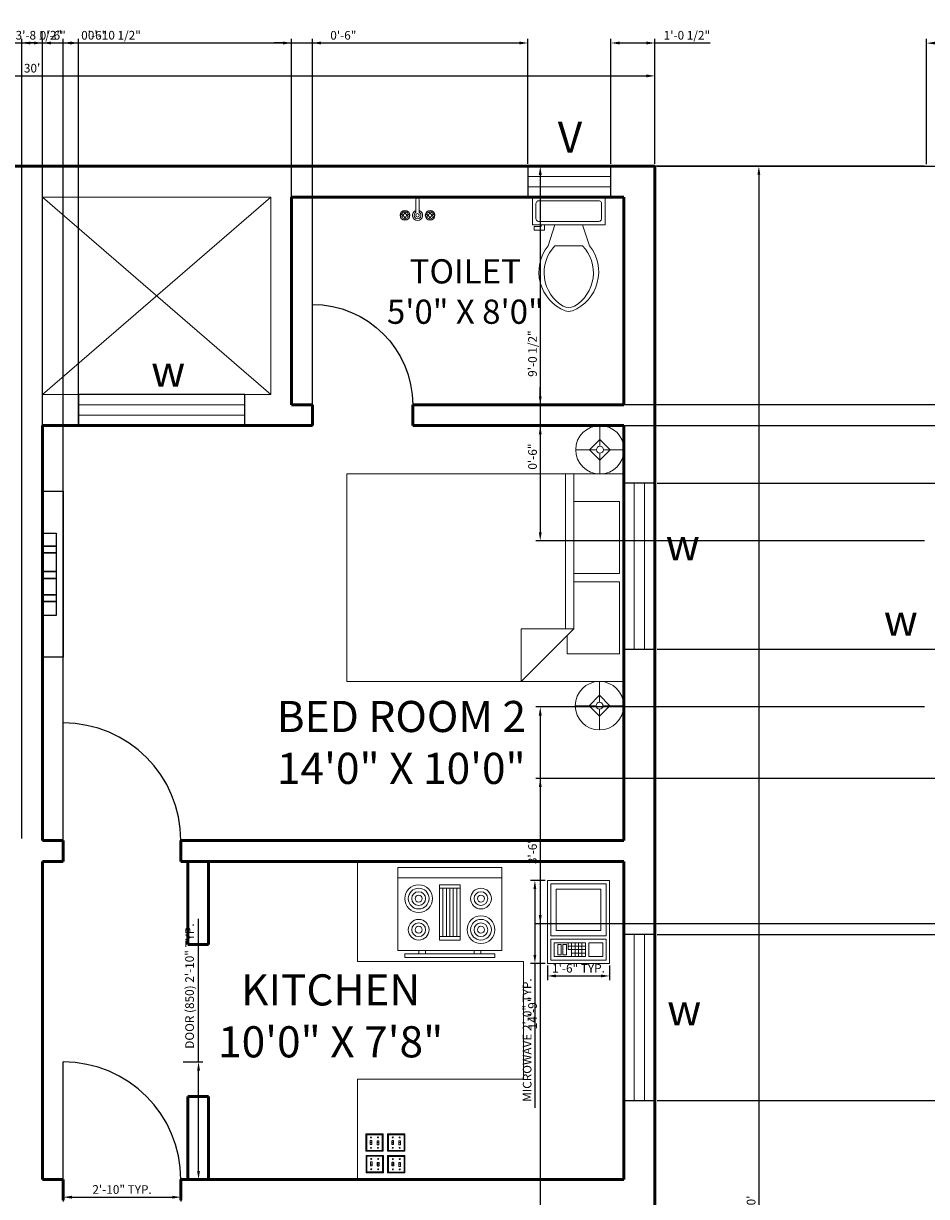
# Model space of a CAD drawing. Units: inches. Extents: x 3688 to 4628, y 1593 to 2337.
# Tile 4 of 7: x 3907 to 4168, y 1997 to 2337. Entities that reach past the tile are written whole.
import ezdxf

# ---------------------------------------------------------------- set-up
doc = ezdxf.new("R2010")
doc.units = ezdxf.units.IN
for name, color, linetype, lineweight in [('A-ANNO-DIMS', 2, 'Continuous', 18), ('A-ANNO-TEXT', 7, 'Continuous', 18), ('A-AREA-IDEN', 7, 'Continuous', 25), ('A-DOOR', 4, 'Continuous', 25), ('A-EQPM', 8, 'Continuous', 18), ('A-FLOR-FIXT', 8, 'Continuous', 18), ('A-FLOR-SHFT', 8, 'Continuous', 18), ('A-FURN', 8, 'Continuous', 18), ('A-GLAZ', 4, 'Continuous', 25), ('A-WALL', 7, 'Continuous', 50), ('E-LITE', 6, 'Continuous', 18)]:
    doc.layers.add(name, color=color, linetype=linetype, lineweight=lineweight)
doc.styles.get("Standard").update_dxf_attribs({"font": 'arial.ttf'})
doc.dimstyles.new('ISO-25', dxfattribs={"dimtxt": 2.5, "dimasz": 2.5, "dimexe": 1.25, "dimexo": 0.625, "dimtad": 1, "dimdec": 0, "dimlunit": 3, "dimtxsty": 'Standard', "dimcen": 2.5, "dimadec": 0, "dimazin": 0, "dimtfac": 1, "dimtdec": 0, "dimtmove": 0, "dimatfit": 3, "dimfxl": 1, "dimarcsym": 0})

# ---------------------------------------------------------------- blocks, each defined once
blk = doc.blocks.new('Bed - Queen')
for p, q in [((0, -80.00003), (0, 0)), ((0, 0), (59.99999, 0)), ((59.99999, 0), (59.99999, -80.00003)), ((7.99999, -1.2), (28.79998, -1.2)), ((7.99999, -14.4), (7.99999, -1.2)), ((28.79998, -1.2), (28.79998, -14.4)), ((31.19999, -1.2), (51.99999, -1.2)), ((31.19999, -14.4), (31.19999, -1.2)), ((51.99999, -1.2), (51.99999, -16.4)), ((0, -14.4), (44.8, -14.4)), ((44.8, -16.8), (0, -16.8)), ((59.99999, -29.6), (44.8, -14.4)), ((44.8, -14.4), (44.8, -29.6)), ((51.99999, -16.4), (46.79936, -16.4)), ((44.8, -29.6), (59.99999, -29.6)), ((59.99999, -80.00003), (0, -80.00003))]:
    blk.add_line(p, q)
blk = doc.blocks.new('Lamp - Table')
for p, q in [((0, 7), (0, 1)), ((-1, 0), (-7, 0)), ((0, 3), (-3, 0)), ((-3, 0), (0, -3)), ((3, 0), (0, 3)), ((0, -3), (3, 0)), ((1, 0), (7, 0)), ((0, -1), (0, -7))]:
    blk.add_line(p, q)
for radius in [7, 1]:
    blk.add_circle((0, 0), radius)
blk = doc.blocks.new('Toilet - top')
for p, q in [((9.5, -6), (9.5, -2)), ((-10, -8.5), (-8, -8.5)), ((-10, -9.5), (-10, -8.5)), ((-7, -9.5), (-10, -9.5)), ((-8, -8.5), (-8, -8)), ((-7, -8), (-7, -9.5)), ((-4, -8), (-6, -14)), ((4, -8), (6, -14)), ((4, -14), (-4, -14))]:
    blk.add_line(p, q)
blk.add_lwpolyline([(10.5, -8), (10.5, 0), (-10.5, 0), (-10.5, -8)], close=True)
for points in [[(-9.5, -2), (-9.5, -6)], [(8.5, -1), (-8.5, -1)], [(-8.5, -7), (8.5, -7)]]:
    blk.add_lwpolyline(points)
for centre, radius, start, end in [((-8.62, -1.88), 0.884, 81.8699, 188.1301), ((8.62, -1.88), 0.884, 351.8699, 98.1301), ((-8.62, -6.12), 0.884, 171.8699, 278.1301), ((8.62, -6.12), 0.884, 261.8699, 8.1301), ((3.52, -21.58), 12.17, 141.4691, 247.9714), ((4.2, -21.82), 11.33, 136.3677, 238.9468), ((-3.52, -21.58), 12.17, 292.0284, 38.5307), ((-4.2, -21.82), 11.33, 301.053, 43.6321), ((0, -27.88), 4, 245.7318, 294.2682), ((0, -29), 4, 254.8605, 285.1395)]:
    blk.add_arc(centre, radius, start, end)
blk = doc.blocks.new('Range-Oven - 30 in top')
for p, q in [((0, -3), (30, -3)), ((12, -6), (18, -6)), ((13, -20), (13, -6)), ((14, -6), (14, -20)), ((15, -20), (15, -6)), ((16, -6), (16, -20)), ((17, -20), (17, -6)), ((18, -20), (12, -20)), ((6, -24), (6, -25)), ((8, -25), (8, -24)), ((22, -25), (22, -24)), ((24, -24), (24, -25))]:
    blk.add_line(p, q)
for points in [[(0, -24), (0, 0), (30, 0), (30, -24)], [(12, -21), (12, -5), (18, -5), (18, -21)], [(2, -26), (2, -25), (28, -25), (28, -26)]]:
    blk.add_lwpolyline(points, close=True)
for centre, radius in [((6, -9), 4), ((6, -9), 3), ((24, -9), 3), ((6, -9), 2), ((6, -9), 1), ((24, -9), 2), ((24, -9), 1), ((6, -18), 3), ((6, -18), 2), ((24, -18), 4), ((24, -18), 3), ((24, -18), 2), ((6, -18), 1), ((24, -18), 1)]:
    blk.add_circle(centre, radius)
blk = doc.blocks.new('Microwave')
for p, q in [((19, 7), (19, 11)), ((20, 11), (20, 7)), ((21, 7), (21, 11)), ((18, 10), (22, 10)), ((22, 9), (18, 9)), ((18, 8), (22, 8)), ((22, 7), (18, 7)), ((19, 6), (19, 7)), ((20, 7), (20, 6)), ((20, 6), (18, 6))]:
    blk.add_line(p, q)
for points in [[(0, 0), (0, 18), (24, 18), (24, 0)], [(1, 1), (1, 17), (16, 17), (16, 1)], [(17, 1), (17, 17), (23, 17), (23, 1)], [(2.5, 2.5), (2.5, 15.5), (14.5, 15.5), (14.5, 2.5)], [(18, 12), (18, 16), (22, 16), (22, 12)], [(18, 2), (18, 11), (22, 11), (22, 2)], [(18.5, 4.5), (18.5, 5.5), (21.5, 5.5), (21.5, 4.5)], [(18.5, 3), (18.5, 4), (21.5, 4), (21.5, 3)]]:
    blk.add_lwpolyline(points, close=True)
blk = doc.blocks.new('Light Switch - Dual')
for p, q in [((-2.25, 4.75), (-2.5, 5)), ((-2.25, 4.75), (2.25, 4.75)), ((-2.25, 0.25), (-2.25, 4.75)), ((-0.875, 4), (-1.125, 4)), ((0.875, 4), (1.125, 4)), ((2.25, 4.75), (2.5, 5)), ((2.25, 4.75), (2.25, 0.25)), ((-2.25, 0.25), (-2.5, 0)), ((2.25, 0.25), (-2.25, 0.25)), ((-0.7854, 2.5), (-1.2183, 2.5)), ((-0.875, 1), (-1.125, 1)), ((0.7854, 2.5), (1.2182, 2.5)), ((0.875, 1), (1.125, 1)), ((2.25, 0.25), (2.5, 0))]:
    blk.add_line(p, q)
for points in [[(-2.5, 0), (-2.5, 5), (2.5, 5), (2.5, 0)], [(-0.78, 3.125), (-0.78, 2), (-1.22, 2), (-1.22, 3.125)], [(0.78, 1.875), (0.78, 3), (1.22, 3), (1.22, 1.875)]]:
    blk.add_lwpolyline(points, close=True)
for points in [[(-0.7818, 3), (-0.75, 3), (-0.75, 2), (-1.25, 2), (-1.25, 3), (-1.2219, 3)], [(0.7817, 2), (0.75, 2), (0.75, 3), (1.25, 3), (1.25, 2), (1.2219, 2)]]:
    blk.add_lwpolyline(points)
for centre in [(-1, 4), (1, 4), (-1, 1), (1, 1)]:
    blk.add_circle(centre, 0.125)
blk = doc.blocks.new('Faucet - Bathroom top')
for p, q in [((-4.107, 0.125), (-4.375, 0.125)), ((-3.75, 0.4788), (-3.75, 0.75)), ((-3.5, 0.482), (-3.5, 0.75)), ((-3.1461, 0.125), (-2.875, 0.125)), ((3.143, 0.125), (2.875, 0.125)), ((3.5, 0.4788), (3.5, 0.75)), ((3.75, 0.482), (3.75, 0.75)), ((4.1039, 0.125), (4.375, 0.125)), ((-4.1039, -0.125), (-4.375, -0.125)), ((-3.75, -0.4821), (-3.75, -0.75)), ((-3.5, -0.4789), (-3.5, -0.75)), ((-3.143, -0.125), (-2.875, -0.125)), ((-0.5, -0.8639), (-0.5, -4.5)), ((0.5, -4.5), (0.5, -0.8631)), ((3.1461, -0.125), (2.875, -0.125)), ((3.5, -0.4821), (3.5, -0.75)), ((3.75, -0.4789), (3.75, -0.75)), ((4.107, -0.125), (4.375, -0.125))]:
    blk.add_line(p, q)
for centre, radius in [((-3.625, 0), 1.375), ((-4.625, 0), 0.2795), ((-3.625, 0), 0.5), ((-3.625, 1), 0.2795), ((-2.625, 0), 0.2795), ((0, 0), 0.5), ((3.625, 0), 1.375), ((2.625, 0), 0.2795), ((3.625, 0), 0.5), ((3.625, 1), 0.2795), ((4.625, 0), 0.2795), ((-3.625, -1), 0.2795), ((3.625, -1), 0.2795)]:
    blk.add_circle(centre, radius)
for centre, radius, start, end in [((-3.625, 0), 1, 105.2407, 164.2093), ((-3.625, 0), 1, 16.44125, 74.07887), ((0, 0), 1.5, 289.6514, 250.3603), ((0, 0), 1, 300.3431, 239.7554), ((3.625, 0), 1, 106.12, 164.0884), ((3.625, 0), 1, 16.23422, 73.90469), ((-3.625, 0), 1, 196.2342, 253.9047), ((-3.625, 0), 1, 286.12, 344.0884), ((3.625, 0), 1, 196.4413, 254.0789), ((3.625, 0), 1, 285.2407, 344.2093), ((0, -4.5), 0.5, 180, 0)]:
    blk.add_arc(centre, radius, start, end)
blk = doc.blocks.new('*D16')
at = {"layer": 'A-ANNO-DIMS', "color": 0, "lineweight": -2, "transparency": 16777216}
for p, q in [((3729.62, 2295.94), (3729.62, 2322.66)), ((3732.12, 2321.41), (4087.12, 2321.41)), ((4089.62, 2295.94), (4089.62, 2322.66))]:
    blk.add_line(p, q, dxfattribs=at)
at = {"layer": 'A-ANNO-DIMS', "color": 0, "transparency": 16777216}
for points in [[(3732.12, 2321.83), (3732.12, 2320.99), (3729.62, 2321.41)], [(4087.12, 2321.83), (4087.12, 2320.99), (4089.62, 2321.41)]]:
    blk.add_solid(points, dxfattribs=at)
at = {"layer": 'Defpoints', "color": 0, "transparency": 16777216}
for p in [(4089.62, 2321.41), (3729.62, 2295.32), (4089.62, 2295.32)]:
    blk.add_point(p, dxfattribs=at)
at = {"layer": 'A-ANNO-DIMS', "color": 0, "transparency": 16777216, "insert": (3909.62, 2323.31), "char_height": 2.5, "attachment_point": 5}
blk.add_mtext("30'", dxfattribs=at)
blk = doc.blocks.new('*D17')
at = {"layer": 'A-ANNO-DIMS', "color": 0, "lineweight": -2, "transparency": 16777216}
for p, q in [((4090.25, 2295.32), (4120.92, 2295.32)), ((4119.67, 2292.82), (4119.67, 1697.82)), ((4090.25, 1695.32), (4120.92, 1695.32))]:
    blk.add_line(p, q, dxfattribs=at)
at = {"layer": 'A-ANNO-DIMS', "color": 0, "transparency": 16777216}
for points in [[(4119.25, 2292.82), (4120.08, 2292.82), (4119.67, 2295.32)], [(4119.25, 1697.82), (4120.08, 1697.82), (4119.67, 1695.32)]]:
    blk.add_solid(points, dxfattribs=at)
at = {"layer": 'Defpoints', "color": 0, "transparency": 16777216}
for p in [(4089.62, 2295.32), (4089.62, 1695.32), (4119.67, 1695.32)]:
    blk.add_point(p, dxfattribs=at)
at = {"layer": 'A-ANNO-DIMS', "color": 0, "transparency": 16777216, "insert": (4117.76, 1995.32), "char_height": 2.5, "attachment_point": 5, "rotation": 90}
blk.add_mtext("50'", dxfattribs=at)
blk = doc.blocks.new('DOOR-850')
blk.add_line((0, 0), (0, 34))
blk.add_arc((0, 0), 34, 0, 90)
blk = doc.blocks.new('DOOR-750')
blk.add_line((29, 0), (29, 29))
blk.add_arc((29, 0), 29, 90, 180)
blk = doc.blocks.new('WIN-1200')
for p, q in [((0, 48), (0, 0)), ((9, 48), (0, 48)), ((9, 0), (9, 48)), ((0, 0), (9, 0))]:
    blk.add_line(p, q)
blk = doc.blocks.new('WIN-600')
for p, q in [((24, 9), (0, 9)), ((0, 9), (0, 0)), ((24, 0), (24, 9)), ((0, 0), (24, 0))]:
    blk.add_line(p, q)
blk = doc.blocks.new('*D29')
at = {"layer": 'A-ANNO-DIMS', "color": 0, "lineweight": -2, "transparency": 16777216}
for p, q in [((3957.72, 2036.32), (3957.72, 2077.7)), ((3953.25, 2036.32), (3958.97, 2036.32)), ((3957.72, 2004.82), (3957.72, 2033.82)), ((3953.25, 2002.32), (3958.97, 2002.32))]:
    blk.add_line(p, q, dxfattribs=at)
at = {"layer": 'A-ANNO-DIMS', "color": 0, "transparency": 16777216}
for points in [[(3957.31, 2033.82), (3958.14, 2033.82), (3957.72, 2036.32)], [(3957.31, 2004.82), (3958.14, 2004.82), (3957.72, 2002.32)]]:
    blk.add_solid(points, dxfattribs=at)
at = {"layer": 'Defpoints', "color": 0, "transparency": 16777216}
for p in [(3952.62, 2036.32), (3957.72, 2036.32), (3952.62, 2002.32)]:
    blk.add_point(p, dxfattribs=at)
at = {"layer": 'A-ANNO-DIMS', "color": 0, "transparency": 16777216, "insert": (3955.46, 2058.26), "char_height": 2.5, "attachment_point": 5, "rotation": 90}
blk.add_mtext('DOOR (850) 2\'-10" TYP.', dxfattribs=at)
blk = doc.blocks.new('*D30')
at = {"layer": 'A-ANNO-DIMS', "color": 0, "lineweight": -2, "transparency": 16777216}
for p, q in [((3918.62, 2001.69), (3918.62, 1995.97)), ((3952.62, 2001.69), (3952.62, 1995.97)), ((3921.12, 1997.22), (3950.12, 1997.22))]:
    blk.add_line(p, q, dxfattribs=at)
at = {"layer": 'A-ANNO-DIMS', "color": 0, "transparency": 16777216}
for points in [[(3921.12, 1997.64), (3921.12, 1996.8), (3918.62, 1997.22)], [(3950.12, 1997.64), (3950.12, 1996.8), (3952.62, 1997.22)]]:
    blk.add_solid(points, dxfattribs=at)
at = {"layer": 'Defpoints', "color": 0, "transparency": 16777216}
for p in [(3918.62, 2002.32), (3952.62, 2002.32), (3952.62, 1997.22)]:
    blk.add_point(p, dxfattribs=at)
at = {"layer": 'A-ANNO-DIMS', "color": 0, "transparency": 16777216, "insert": (3935.62, 1999.12), "char_height": 2.5, "attachment_point": 5}
blk.add_mtext('2\'-10" TYP.', dxfattribs=at)
blk = doc.blocks.new('*D43')
at = {"layer": 'A-ANNO-DIMS', "color": 0, "lineweight": -2, "transparency": 16777216}
for p, q in [((4057.91, 2088.79), (4053.69, 2088.79)), ((4054.94, 2086.29), (4054.94, 2067.29)), ((4057.91, 2064.79), (4053.69, 2064.79)), ((4054.94, 2064.79), (4054.94, 2023.02))]:
    blk.add_line(p, q, dxfattribs=at)
at = {"layer": 'A-ANNO-DIMS', "color": 0, "transparency": 16777216}
for points in [[(4054.52, 2086.29), (4055.35, 2086.29), (4054.94, 2088.79)], [(4054.52, 2067.29), (4055.35, 2067.29), (4054.94, 2064.79)]]:
    blk.add_solid(points, dxfattribs=at)
at = {"layer": 'Defpoints', "color": 0, "transparency": 16777216}
for p in [(4058.54, 2088.79), (4054.94, 2064.79), (4058.54, 2064.79)]:
    blk.add_point(p, dxfattribs=at)
at = {"layer": 'A-ANNO-DIMS', "color": 0, "transparency": 16777216, "insert": (4053.02, 2042.65), "char_height": 2.5, "attachment_point": 5, "rotation": 90}
blk.add_mtext('MICROWAVE 2\'-0" TYP.', dxfattribs=at)
blk = doc.blocks.new('*D44')
at = {"layer": 'A-ANNO-DIMS', "color": 0, "lineweight": -2, "transparency": 16777216}
for p, q in [((4058.54, 2064.16), (4058.54, 2059.94)), ((4076.54, 2064.16), (4076.54, 2059.94)), ((4061.04, 2061.19), (4074.04, 2061.19))]:
    blk.add_line(p, q, dxfattribs=at)
at = {"layer": 'A-ANNO-DIMS', "color": 0, "transparency": 16777216}
for points in [[(4061.04, 2061.6), (4061.04, 2060.77), (4058.54, 2061.19)], [(4074.04, 2061.6), (4074.04, 2060.77), (4076.54, 2061.19)]]:
    blk.add_solid(points, dxfattribs=at)
at = {"layer": 'Defpoints', "color": 0, "transparency": 16777216}
for p in [(4058.54, 2064.79), (4076.54, 2064.79), (4076.54, 2061.19)]:
    blk.add_point(p, dxfattribs=at)
at = {"layer": 'A-ANNO-DIMS', "color": 0, "transparency": 16777216, "insert": (4067.54, 2063.09), "char_height": 2.5, "attachment_point": 5}
blk.add_mtext('1\'-6" TYP.', dxfattribs=at)
blk = doc.blocks.new('*D57')
at = {"layer": 'A-ANNO-DIMS', "color": 0, "lineweight": -2, "transparency": 16777216}
for p, q in [((4090.25, 2295.32), (4188.4, 2295.32)), ((4187.15, 2292.82), (4187.15, 2206.19)), ((4090.25, 2203.69), (4188.4, 2203.69))]:
    blk.add_line(p, q, dxfattribs=at)
at = {"layer": 'A-ANNO-DIMS', "color": 0, "transparency": 16777216}
for points in [[(4186.74, 2292.82), (4187.57, 2292.82), (4187.15, 2295.32)], [(4186.74, 2206.19), (4187.57, 2206.19), (4187.15, 2203.69)]]:
    blk.add_solid(points, dxfattribs=at)
at = {"layer": 'Defpoints', "color": 0, "transparency": 16777216}
for p in [(4089.62, 2295.32), (4089.62, 2203.69), (4187.15, 2203.69)]:
    blk.add_point(p, dxfattribs=at)
at = {"layer": 'A-ANNO-DIMS', "color": 0, "transparency": 16777216, "insert": (4185.24, 2249.51), "char_height": 2.5, "attachment_point": 5, "rotation": 90}
blk.add_mtext('7\'-7 1/2"', dxfattribs=at)
blk = doc.blocks.new('*D58')
at = {"layer": 'A-ANNO-DIMS', "color": 0, "lineweight": -2, "transparency": 16777216}
for p, q in [((4090.25, 2155.69), (4188.4, 2155.69)), ((4187.15, 2153.19), (4187.15, 2075.67)), ((4090.25, 2073.17), (4188.4, 2073.17))]:
    blk.add_line(p, q, dxfattribs=at)
at = {"layer": 'A-ANNO-DIMS', "color": 0, "transparency": 16777216}
for points in [[(4186.74, 2153.19), (4187.57, 2153.19), (4187.15, 2155.69)], [(4186.74, 2075.67), (4187.57, 2075.67), (4187.15, 2073.17)]]:
    blk.add_solid(points, dxfattribs=at)
at = {"layer": 'Defpoints', "color": 0, "transparency": 16777216}
for p in [(4089.62, 2155.69), (4089.62, 2073.17), (4187.15, 2073.17)]:
    blk.add_point(p, dxfattribs=at)
at = {"layer": 'A-ANNO-DIMS', "color": 0, "transparency": 16777216, "insert": (4185.24, 2114.43), "char_height": 2.5, "attachment_point": 5, "rotation": 90}
blk.add_mtext('6\'-10 1/2"', dxfattribs=at)
blk = doc.blocks.new('*D59')
at = {"layer": 'A-ANNO-DIMS', "color": 0, "lineweight": -2, "transparency": 16777216}
for p, q in [((4090.25, 2025.17), (4188.4, 2025.17)), ((4187.15, 2022.67), (4187.15, 1991.6)), ((4090.25, 1989.1), (4188.4, 1989.1))]:
    blk.add_line(p, q, dxfattribs=at)
at = {"layer": 'A-ANNO-DIMS', "color": 0, "transparency": 16777216}
for points in [[(4186.74, 2022.67), (4187.57, 2022.67), (4187.15, 2025.17)], [(4186.74, 1991.6), (4187.57, 1991.6), (4187.15, 1989.1)]]:
    blk.add_solid(points, dxfattribs=at)
at = {"layer": 'Defpoints', "color": 0, "transparency": 16777216}
for p in [(4089.62, 2025.17), (4089.62, 1989.1), (4187.15, 1989.1)]:
    blk.add_point(p, dxfattribs=at)
at = {"layer": 'A-ANNO-DIMS', "color": 0, "transparency": 16777216, "insert": (4185.25, 2007.14), "char_height": 2.5, "attachment_point": 5, "rotation": 90}
blk.add_mtext('3\'-0"', dxfattribs=at)
blk = doc.blocks.new('*D63')
at = {"layer": 'A-ANNO-DIMS', "color": 0, "lineweight": -2, "transparency": 16777216}
for p, q in [((3768.3, 2295.94), (3768.3, 2332.17)), ((3770.8, 2330.92), (4050.42, 2330.92)), ((4052.92, 2295.94), (4052.92, 2332.17))]:
    blk.add_line(p, q, dxfattribs=at)
at = {"layer": 'A-ANNO-DIMS', "color": 0, "transparency": 16777216}
for points in [[(3770.8, 2331.34), (3770.8, 2330.5), (3768.3, 2330.92)], [(4050.42, 2331.34), (4050.42, 2330.5), (4052.92, 2330.92)]]:
    blk.add_solid(points, dxfattribs=at)
at = {"layer": 'Defpoints', "color": 0, "transparency": 16777216}
for p in [(4052.92, 2330.92), (3768.3, 2295.32), (4052.92, 2295.32)]:
    blk.add_point(p, dxfattribs=at)
at = {"layer": 'A-ANNO-DIMS', "color": 0, "transparency": 16777216, "insert": (3910.61, 2332.84), "char_height": 2.5, "attachment_point": 5}
blk.add_mtext('23\'-8 1/2"', dxfattribs=at)
blk = doc.blocks.new('*D64')
at = {"layer": 'A-ANNO-DIMS', "color": 0, "lineweight": -2, "transparency": 16777216}
for p, q in [((4076.92, 2295.94), (4076.92, 2332.17)), ((4079.42, 2330.92), (4087.12, 2330.92)), ((4089.62, 2295.94), (4089.62, 2332.17)), ((4089.62, 2330.92), (4105.61, 2330.92))]:
    blk.add_line(p, q, dxfattribs=at)
at = {"layer": 'A-ANNO-DIMS', "color": 0, "transparency": 16777216}
for points in [[(4079.42, 2331.34), (4079.42, 2330.5), (4076.92, 2330.92)], [(4087.12, 2331.34), (4087.12, 2330.5), (4089.62, 2330.92)]]:
    blk.add_solid(points, dxfattribs=at)
at = {"layer": 'Defpoints', "color": 0, "transparency": 16777216}
for p in [(4089.62, 2330.92), (4076.92, 2295.32), (4089.62, 2295.32)]:
    blk.add_point(p, dxfattribs=at)
at = {"layer": 'A-ANNO-DIMS', "color": 0, "transparency": 16777216, "insert": (4098.87, 2332.84), "char_height": 2.5, "attachment_point": 5}
blk.add_mtext('1\'-0 1/2"', dxfattribs=at)
blk = doc.blocks.new('*D66')
at = {"layer": 'A-ANNO-DIMS', "color": 0, "lineweight": -2, "transparency": 16777216}
for p, q in [((3912.62, 2220.94), (3912.62, 2332.17)), ((3915.12, 2330.92), (3920.56, 2330.92)), ((3923.06, 2220.94), (3923.06, 2332.17)), ((3923.06, 2330.92), (3941.22, 2330.92))]:
    blk.add_line(p, q, dxfattribs=at)
at = {"layer": 'A-ANNO-DIMS', "color": 0, "transparency": 16777216}
for points in [[(3915.12, 2331.34), (3915.12, 2330.5), (3912.62, 2330.92)], [(3920.56, 2331.34), (3920.56, 2330.5), (3923.06, 2330.92)]]:
    blk.add_solid(points, dxfattribs=at)
at = {"layer": 'Defpoints', "color": 0, "transparency": 16777216}
for p in [(3923.06, 2330.92), (3912.62, 2220.32), (3923.06, 2220.32)]:
    blk.add_point(p, dxfattribs=at)
at = {"layer": 'A-ANNO-DIMS', "color": 0, "transparency": 16777216, "insert": (3933.39, 2332.84), "char_height": 2.5, "attachment_point": 5}
blk.add_mtext('0\'-10 1/2"', dxfattribs=at)
blk = doc.blocks.new('*D68')
at = {"layer": 'A-ANNO-DIMS', "color": 0, "lineweight": -2, "transparency": 16777216}
for p, q in [((3982.12, 2330.92), (3979.62, 2330.92)), ((3984.62, 2226.94), (3984.62, 2332.17)), ((3984.62, 2330.92), (3990.62, 2330.92)), ((3990.62, 2226.94), (3990.62, 2332.17)), ((3993.12, 2330.92), (4003.52, 2330.92))]:
    blk.add_line(p, q, dxfattribs=at)
at = {"layer": 'A-ANNO-DIMS', "color": 0, "transparency": 16777216}
for points in [[(3982.12, 2331.34), (3982.12, 2330.5), (3984.62, 2330.92)], [(3993.12, 2331.34), (3993.12, 2330.5), (3990.62, 2330.92)]]:
    blk.add_solid(points, dxfattribs=at)
at = {"layer": 'Defpoints', "color": 0, "transparency": 16777216}
for p in [(3990.62, 2330.92), (3984.62, 2226.32), (3990.62, 2226.32)]:
    blk.add_point(p, dxfattribs=at)
at = {"layer": 'A-ANNO-DIMS', "color": 0, "transparency": 16777216, "insert": (3999.57, 2332.82), "char_height": 2.5, "attachment_point": 5}
blk.add_mtext('0\'-6"', dxfattribs=at)
blk = doc.blocks.new('*D70')
at = {"layer": 'A-ANNO-DIMS', "color": 0, "lineweight": -2, "transparency": 16777216}
for p, q in [((3898.12, 2330.92), (3895.62, 2330.92)), ((3900.62, 2100.94), (3900.62, 2332.17)), ((3900.62, 2330.92), (3906.62, 2330.92)), ((3906.62, 2100.94), (3906.62, 2332.17)), ((3909.12, 2330.92), (3919.52, 2330.92))]:
    blk.add_line(p, q, dxfattribs=at)
at = {"layer": 'A-ANNO-DIMS', "color": 0, "transparency": 16777216}
for points in [[(3898.12, 2331.34), (3898.12, 2330.5), (3900.62, 2330.92)], [(3909.12, 2331.34), (3909.12, 2330.5), (3906.62, 2330.92)]]:
    blk.add_solid(points, dxfattribs=at)
at = {"layer": 'Defpoints', "color": 0, "transparency": 16777216}
for p in [(3906.62, 2330.92), (3900.62, 2100.32), (3906.62, 2100.32)]:
    blk.add_point(p, dxfattribs=at)
at = {"layer": 'A-ANNO-DIMS', "color": 0, "transparency": 16777216, "insert": (3915.57, 2332.82), "char_height": 2.5, "attachment_point": 5}
blk.add_mtext('0\'-6"', dxfattribs=at)
blk = doc.blocks.new('*D71')
at = {"layer": 'A-ANNO-DIMS', "color": 0, "lineweight": -2, "transparency": 16777216}
for p, q in [((3910.12, 2330.92), (3907.62, 2330.92)), ((3912.62, 2100.94), (3912.62, 2332.17)), ((3912.62, 2330.92), (3918.62, 2330.92)), ((3918.62, 2100.94), (3918.62, 2332.17)), ((3921.12, 2330.92), (3931.52, 2330.92))]:
    blk.add_line(p, q, dxfattribs=at)
at = {"layer": 'A-ANNO-DIMS', "color": 0, "transparency": 16777216}
for points in [[(3910.12, 2331.34), (3910.12, 2330.5), (3912.62, 2330.92)], [(3921.12, 2331.34), (3921.12, 2330.5), (3918.62, 2330.92)]]:
    blk.add_solid(points, dxfattribs=at)
at = {"layer": 'Defpoints', "color": 0, "transparency": 16777216}
for p in [(3918.62, 2330.92), (3912.62, 2100.32), (3918.62, 2100.32)]:
    blk.add_point(p, dxfattribs=at)
at = {"layer": 'A-ANNO-DIMS', "color": 0, "transparency": 16777216, "insert": (3927.57, 2332.82), "char_height": 2.5, "attachment_point": 5}
blk.add_mtext('0\'-6"', dxfattribs=at)
blk = doc.blocks.new('*D80')
at = {"layer": 'A-ANNO-DIMS', "color": 0, "lineweight": -2, "transparency": 16777216}
for p, q in [((4167.51, 2295.28), (4055.24, 2295.28)), ((4056.49, 2292.78), (4056.49, 2189.46)), ((4167.51, 2186.96), (4055.24, 2186.96))]:
    blk.add_line(p, q, dxfattribs=at)
at = {"layer": 'A-ANNO-DIMS', "color": 0, "transparency": 16777216}
for points in [[(4056.07, 2292.78), (4056.9, 2292.78), (4056.49, 2295.28)], [(4056.07, 2189.46), (4056.9, 2189.46), (4056.49, 2186.96)]]:
    blk.add_solid(points, dxfattribs=at)
at = {"layer": 'Defpoints', "color": 0, "transparency": 16777216}
for p in [(4168.13, 2295.28), (4056.49, 2186.96), (4168.13, 2186.96)]:
    blk.add_point(p, dxfattribs=at)
at = {"layer": 'A-ANNO-DIMS', "color": 0, "transparency": 16777216, "insert": (4054.57, 2241.12), "char_height": 2.5, "attachment_point": 5, "rotation": 90}
blk.add_mtext('9\'-0 1/2"', dxfattribs=at)
blk = doc.blocks.new('*D81')
at = {"layer": 'A-ANNO-DIMS', "color": 0, "lineweight": -2, "transparency": 16777216}
for p, q in [((4167.51, 2138.96), (4055.24, 2138.96)), ((4056.49, 2136.46), (4056.49, 1964.52)), ((4167.51, 1962.02), (4055.24, 1962.02))]:
    blk.add_line(p, q, dxfattribs=at)
at = {"layer": 'A-ANNO-DIMS', "color": 0, "transparency": 16777216}
for points in [[(4056.07, 2136.46), (4056.9, 2136.46), (4056.49, 2138.96)], [(4056.07, 1964.52), (4056.9, 1964.52), (4056.49, 1962.02)]]:
    blk.add_solid(points, dxfattribs=at)
at = {"layer": 'Defpoints', "color": 0, "transparency": 16777216}
for p in [(4168.13, 2138.96), (4056.49, 1962.02), (4168.13, 1962.02)]:
    blk.add_point(p, dxfattribs=at)
at = {"layer": 'A-ANNO-DIMS', "color": 0, "transparency": 16777216, "insert": (4054.58, 2050.49), "char_height": 2.5, "attachment_point": 5, "rotation": 90}
blk.add_mtext('14\'-9"', dxfattribs=at)
blk = doc.blocks.new('*D89')
at = {"layer": 'A-ANNO-DIMS', "color": 0, "lineweight": -2, "transparency": 16777216}
for p, q in [((4168.13, 2295.91), (4168.13, 2332.13)), ((4170.63, 2330.88), (4185.49, 2330.88)), ((4187.99, 2295.91), (4187.99, 2332.13))]:
    blk.add_line(p, q, dxfattribs=at)
at = {"layer": 'A-ANNO-DIMS', "color": 0, "transparency": 16777216}
for points in [[(4170.63, 2331.3), (4170.63, 2330.47), (4168.13, 2330.88)], [(4185.49, 2331.3), (4185.49, 2330.47), (4187.99, 2330.88)]]:
    blk.add_solid(points, dxfattribs=at)
at = {"layer": 'Defpoints', "color": 0, "transparency": 16777216}
for p in [(4187.99, 2330.88), (4168.13, 2295.28), (4187.99, 2295.28)]:
    blk.add_point(p, dxfattribs=at)
at = {"layer": 'A-ANNO-DIMS', "color": 0, "transparency": 16777216, "insert": (4178.06, 2332.78), "char_height": 2.5, "attachment_point": 5}
blk.add_mtext('1\'-8"', dxfattribs=at)
blk = doc.blocks.new('*D94')
at = {"layer": 'A-ANNO-DIMS', "color": 0, "lineweight": -2, "transparency": 16777216}
for p, q in [((4056.49, 2228.78), (4056.49, 2231.28)), ((4237.51, 2226.28), (4055.24, 2226.28)), ((4056.49, 2226.28), (4056.49, 2220.28)), ((4237.51, 2220.28), (4055.24, 2220.28)), ((4056.49, 2217.78), (4056.49, 2207.39))]:
    blk.add_line(p, q, dxfattribs=at)
at = {"layer": 'A-ANNO-DIMS', "color": 0, "transparency": 16777216}
for points in [[(4056.07, 2228.78), (4056.9, 2228.78), (4056.49, 2226.28)], [(4056.07, 2217.78), (4056.9, 2217.78), (4056.49, 2220.28)]]:
    blk.add_solid(points, dxfattribs=at)
at = {"layer": 'Defpoints', "color": 0, "transparency": 16777216}
for p in [(4238.13, 2226.28), (4056.49, 2220.28), (4238.13, 2220.28)]:
    blk.add_point(p, dxfattribs=at)
at = {"layer": 'A-ANNO-DIMS', "color": 0, "transparency": 16777216, "insert": (4054.58, 2211.34), "char_height": 2.5, "attachment_point": 5, "rotation": 90}
blk.add_mtext('0\'-6"', dxfattribs=at)
blk = doc.blocks.new('*D96')
at = {"layer": 'A-ANNO-DIMS', "color": 0, "lineweight": -2, "transparency": 16777216}
for p, q in [((4320.51, 2118.28), (4055.24, 2118.28)), ((4056.49, 2115.78), (4056.49, 2078.78)), ((4320.51, 2076.28), (4055.24, 2076.28))]:
    blk.add_line(p, q, dxfattribs=at)
at = {"layer": 'A-ANNO-DIMS', "color": 0, "transparency": 16777216}
for points in [[(4056.07, 2115.78), (4056.9, 2115.78), (4056.49, 2118.28)], [(4056.07, 2078.78), (4056.9, 2078.78), (4056.49, 2076.28)]]:
    blk.add_solid(points, dxfattribs=at)
at = {"layer": 'Defpoints', "color": 0, "transparency": 16777216}
for p in [(4321.13, 2118.28), (4056.49, 2076.28), (4321.13, 2076.28)]:
    blk.add_point(p, dxfattribs=at)
at = {"layer": 'A-ANNO-DIMS', "color": 0, "transparency": 16777216, "insert": (4054.58, 2097.28), "char_height": 2.5, "attachment_point": 5, "rotation": 90}
blk.add_mtext('3\'-6"', dxfattribs=at)

msp = doc.modelspace()

# ---------------------------------------------------------------- linework, layer by layer
at = {"layer": 'A-FLOR-FIXT'}
for p, q in [((4003.62, 2094.32), (4003.62, 2065.32)), ((4083.62, 2073.17), (4083.62, 2025.17)), ((4086.62, 2025.17), (4086.62, 2073.17)), ((4003.62, 2065.32), (4051.62, 2065.32)), ((4051.62, 2065.32), (4051.62, 2031.32)), ((4003.62, 2031.32), (4051.62, 2031.32)), ((4003.62, 2031.32), (4003.62, 2002.32))]:
    msp.add_line(p, q, dxfattribs=at)
at = {"layer": 'A-FLOR-SHFT'}
for p, q in [((3912.62, 2229.32), (3912.62, 2286.32)), ((3912.62, 2286.32), (3978.62, 2286.32)), ((3978.62, 2286.32), (3912.62, 2229.32)), ((3912.62, 2229.32), (3912.62, 2286.32)), ((3912.62, 2286.32), (3978.62, 2229.32)), ((3978.62, 2286.32), (3978.62, 2229.32)), ((3912.62, 2229.32), (3978.62, 2229.32)), ((3971.06, 2226.32), (3923.06, 2226.32)), ((3923.06, 2223.32), (3971.06, 2223.32))]:
    msp.add_line(p, q, dxfattribs=at)
at = {"layer": 'A-FURN'}
for p, q in [((4076.92, 2292.32), (4052.92, 2292.32)), ((4052.92, 2289.32), (4076.92, 2289.32)), ((4083.62, 2203.69), (4083.62, 2155.69)), ((4086.62, 2155.69), (4086.62, 2203.69))]:
    msp.add_line(p, q, dxfattribs=at)
at = {"layer": 'A-GLAZ'}
for p, q in [((3912.62, 2201.38), (3918.62, 2201.38)), ((3918.62, 2201.38), (3918.62, 2153.38)), ((3912.62, 2189.22), (3916.62, 2189.22)), ((3916.62, 2189.22), (3916.62, 2165.44)), ((3916.62, 2165.44), (3912.62, 2165.44)), ((3918.62, 2153.38), (3912.62, 2153.38))]:
    msp.add_line(p, q, dxfattribs=at)
for points in [[(3912.62, 2185.46), (3916.62, 2185.46), (3916.62, 2185.46), (3912.62, 2185.46)], [(3912.62, 2183.53), (3916.62, 2183.53), (3916.62, 2183.53), (3912.62, 2183.53)], [(3912.62, 2178.08), (3916.62, 2178.08), (3916.62, 2178.08), (3912.62, 2178.08)], [(3912.62, 2176.06), (3916.62, 2176.06), (3916.62, 2176.06), (3912.62, 2176.06)], [(3912.62, 2171.38), (3916.62, 2171.38), (3916.62, 2171.38), (3912.62, 2171.38)], [(3912.62, 2169.49), (3916.62, 2169.49), (3916.62, 2169.49), (3912.62, 2169.49)]]:
    msp.add_lwpolyline(points, close=True, dxfattribs=at)
at = {"layer": 'A-WALL'}
for p, q in [((3729.62, 2295.32), (4089.62, 2295.32)), ((4089.62, 2295.32), (4089.62, 1695.32)), ((3984.62, 2286.32), (3984.62, 2226.32)), ((3984.62, 2286.32), (4080.62, 2286.32)), ((4080.62, 2286.32), (4080.62, 2226.32)), ((3984.62, 2226.32), (3990.62, 2226.32)), ((3984.62, 2226.32), (3990.62, 2226.32)), ((3990.62, 2226.32), (3990.62, 2220.32)), ((4019.62, 2220.32), (4019.62, 2226.32)), ((4019.62, 2226.32), (4080.62, 2226.32)), ((3912.62, 2100.32), (3912.62, 2220.32)), ((3912.62, 2220.32), (3990.62, 2220.32)), ((4019.62, 2220.32), (4080.62, 2220.32)), ((4080.62, 2220.32), (4080.62, 2100.32)), ((3912.62, 2100.32), (3918.62, 2100.32)), ((3912.62, 2100.32), (3918.62, 2100.32)), ((3918.62, 2094.32), (3918.62, 2100.32)), ((3918.62, 2094.32), (3918.62, 2100.32)), ((3952.62, 2100.32), (3952.62, 2094.32)), ((3952.62, 2100.32), (4080.62, 2100.32)), ((3912.62, 2094.32), (3912.62, 2002.32)), ((3912.62, 2094.32), (3918.62, 2094.32)), ((3912.62, 2094.32), (3918.62, 2094.32)), ((3952.62, 2094.32), (3954.62, 2094.32)), ((3954.62, 2094.32), (3954.62, 2070.32)), ((3954.62, 2094.32), (4080.62, 2094.32)), ((3954.62, 2094.32), (3954.62, 2070.32)), ((3954.62, 2094.32), (3954.62, 2070.32)), ((3960.62, 2094.32), (3960.62, 2070.32)), ((4080.62, 2094.32), (4080.62, 2002.32)), ((3954.62, 2070.32), (3960.62, 2070.32)), ((3960.62, 2026.32), (3954.62, 2026.32)), ((3954.62, 2026.32), (3954.62, 2002.32)), ((3954.62, 2026.32), (3954.62, 2002.32)), ((3960.62, 2002.32), (3960.62, 2026.32)), ((3960.62, 2026.32), (3960.62, 2002.32)), ((3912.62, 2002.32), (3918.62, 2002.32)), ((3912.62, 2002.32), (3918.62, 2002.32)), ((3918.62, 2002.32), (3918.62, 1996.32)), ((3954.62, 2002.32), (3952.62, 2002.32)), ((3952.62, 1996.32), (3952.62, 2002.32)), ((3954.62, 2002.32), (4080.62, 2002.32))]:
    msp.add_line(p, q, dxfattribs=at)

# ---------------------------------------------------------------- block references
at = {"layer": 'A-DOOR', "extrusion": (0, 0, -1), "zscale": -1}
msp.add_blockref('DOOR-750', (-4019.62, 2226.32), dxfattribs=at)
at = {"layer": 'A-DOOR'}
for p in [(3918.62, 2100.32), (3918.62, 2002.32)]:
    msp.add_blockref('DOOR-850', p, dxfattribs=at)
at = {"layer": 'A-EQPM'}
msp.add_blockref('Range-Oven - 30 in top', (4015.35, 2092.55), dxfattribs=at)
at = {"layer": 'A-EQPM', "rotation": 270}
msp.add_blockref('Microwave', (4058.54, 2088.79), dxfattribs=at)
at = {"layer": 'A-FLOR-FIXT', "rotation": 180}
msp.add_blockref('Faucet - Bathroom top', (4021.02, 2281.1), dxfattribs=at)
at = {"layer": 'A-FLOR-FIXT'}
msp.add_blockref('Toilet - top', (4064.73, 2286.32), dxfattribs=at)
at = {"layer": 'A-FURN', "rotation": 270}
for name, p in [('Lamp - Table', (4073.73, 2213.32)), ('Bed - Queen', (4080.62, 2206.32)), ('Lamp - Table', (4073.62, 2139.32))]:
    msp.add_blockref(name, p, dxfattribs=at)
at = {"layer": 'A-GLAZ'}
for name, p in [('WIN-600', (4052.92, 2286.32)), ('WIN-1200', (4080.62, 2155.69)), ('WIN-1200', (4080.62, 2025.17))]:
    msp.add_blockref(name, p, dxfattribs=at)
at = {"layer": 'A-GLAZ', "rotation": 270}
msp.add_blockref('WIN-1200', (3923.06, 2229.32), dxfattribs=at)
at = {"layer": 'E-LITE'}
for p in [(4008.57, 2010.5), (4014.86, 2010.5), (4008.65, 2004.29), (4014.88, 2004.25)]:
    msp.add_blockref('Light Switch - Dual', p, dxfattribs=at)

# ---------------------------------------------------------------- texts
at = {"layer": 'A-ANNO-TEXT', "char_height": 9, "attachment_point": 1}
for s, heights, insert in [('\\pxqc;V', [37.18], (3995.84, 2308.19)), ('\\pxqc;w', [0], (3879.71, 2240.56)), ('\\pxqc;w', [0], (4028.44, 2190.38)), ('\\pxqc;w', [0], (4091.46, 2168.59)), ('\\pxqc;w', [0], (4028.86, 2055.89))]:
    msp.add_mtext_dynamic_manual_height_columns(s, width=138.4723, gutter_width=12.5, heights=heights, dxfattribs=dict(at, insert=insert))
at = {"layer": 'A-AREA-IDEN', "attachment_point": 1}
for s, width, insert, char_height in [('\\pxqc;TOILET \\P5\'0" X 8\'0"', 61.3205, (4004.17, 2268.4), 7), ('\\pxqc;BED ROOM 2\\P14\'0" X 10\'0"', 105.0766, (3963.8, 2140.7), 9), ('\\pxqc;KITCHEN^J10\'0" X 7\'8"', 105.0766, (3943.37, 2061.65), 9)]:
    msp.add_mtext_dynamic_manual_height_columns(s, width=width, gutter_width=12.5, heights=[0], dxfattribs=dict(at, insert=insert, char_height=char_height))

# ---------------------------------------------------------------- dimensions: what is measured, and where the dimension line sits
at = {"layer": 'A-ANNO-DIMS'}
for base, p1, p2, override, picture, middle in [((4052.92, 2330.92), (3768.3, 2295.32), (4052.92, 2295.32), {"dimdec": 1, "dimlfac": 1, "dimrnd": 0, "dimzin": 1, "dimdsep": 46, "dimlunit": 4, "dimfrac": 2}, '*D63', (3910.61, 2332.84)), ((3906.62, 2330.92), (3900.62, 2100.32), (3906.62, 2100.32), {"dimdec": 1, "dimlfac": 1, "dimrnd": 0, "dimzin": 1, "dimdsep": 46, "dimlunit": 4, "dimfrac": 2}, '*D70', (3915.57, 2332.82)), ((3918.62, 2330.92), (3912.62, 2100.32), (3918.62, 2100.32), {"dimdec": 1, "dimlfac": 1, "dimrnd": 0, "dimzin": 1, "dimdsep": 46, "dimlunit": 4, "dimfrac": 2}, '*D71', (3927.57, 2332.82)), ((3923.06, 2330.92), (3912.62, 2220.32), (3923.06, 2220.32), {"dimdec": 1, "dimlfac": 1, "dimrnd": 0, "dimzin": 1, "dimdsep": 46, "dimlunit": 4, "dimfrac": 2}, '*D66', (3933.39, 2332.84)), ((3990.62, 2330.92), (3984.62, 2226.32), (3990.62, 2226.32), {"dimdec": 1, "dimlfac": 1, "dimrnd": 0, "dimzin": 1, "dimdsep": 46, "dimlunit": 4, "dimfrac": 2}, '*D68', (3999.57, 2332.82)), ((4089.62, 2330.92), (4076.92, 2295.32), (4089.62, 2295.32), {"dimdec": 1, "dimlfac": 1, "dimrnd": 0, "dimzin": 1, "dimdsep": 46, "dimlunit": 4, "dimfrac": 2}, '*D64', (4098.87, 2332.84)), ((4187.99, 2330.88), (4168.13, 2295.28), (4187.99, 2295.28), {"dimdec": 1, "dimlfac": 1, "dimrnd": 0, "dimzin": 1, "dimdsep": 46, "dimlunit": 4, "dimfrac": 2}, '*D89', (4178.06, 2332.78)), ((4089.62, 2321.41), (3729.62, 2295.32), (4089.62, 2295.32), {"dimclrd": 0, "dimclre": 0, "dimclrt": 0}, '*D16', (3909.62, 2323.31))]:
    dim = msp.add_linear_dim(base=base, p1=p1, p2=p2, dimstyle='ISO-25', override=override, dxfattribs=at)
    dim.commit()
    dim.dimension.update_dxf_attribs({"geometry": picture, "text_midpoint": middle})
for base, p1, p2, override, picture, middle in [((4056.49, 2186.96), (4168.13, 2295.28), (4168.13, 2186.96), {"dimdec": 1, "dimlfac": 1, "dimrnd": 0, "dimzin": 1, "dimdsep": 46, "dimlunit": 4, "dimfrac": 2}, '*D80', (4054.57, 2241.12)), ((4119.67, 1695.32), (4089.62, 2295.32), (4089.62, 1695.32), {"dimclrd": 0, "dimclre": 0, "dimclrt": 0}, '*D17', (4117.76, 1995.32)), ((4187.15, 2203.69), (4089.62, 2295.32), (4089.62, 2203.69), {"dimdec": 1, "dimlfac": 1, "dimrnd": 0, "dimzin": 1, "dimdsep": 46, "dimlunit": 4, "dimfrac": 2}, '*D57', (4185.24, 2249.51)), ((4056.49, 2220.28), (4238.13, 2226.28), (4238.13, 2220.28), {"dimdec": 1, "dimlfac": 1, "dimrnd": 0, "dimzin": 1, "dimdsep": 46, "dimlunit": 4, "dimfrac": 2}, '*D94', (4054.58, 2211.34)), ((4187.15, 2073.17), (4089.62, 2155.69), (4089.62, 2073.17), {"dimdec": 1, "dimlfac": 1, "dimrnd": 0, "dimzin": 1, "dimdsep": 46, "dimlunit": 4, "dimfrac": 2}, '*D58', (4185.24, 2114.43)), ((4056.49, 1962.02), (4168.13, 2138.96), (4168.13, 1962.02), {"dimdec": 1, "dimlfac": 1, "dimrnd": 0, "dimzin": 1, "dimdsep": 46, "dimlunit": 4, "dimfrac": 2}, '*D81', (4054.58, 2050.49)), ((4056.49, 2076.28), (4321.13, 2118.28), (4321.13, 2076.28), {"dimdec": 1, "dimlfac": 1, "dimrnd": 0, "dimzin": 1, "dimdsep": 46, "dimlunit": 4, "dimfrac": 2}, '*D96', (4054.58, 2097.28)), ((4187.15, 1989.1), (4089.62, 2025.17), (4089.62, 1989.1), {"dimdec": 1, "dimlfac": 1, "dimrnd": 0, "dimzin": 1, "dimdsep": 46, "dimlunit": 4, "dimfrac": 2}, '*D59', (4185.25, 2007.14))]:
    dim = msp.add_linear_dim(base=base, p1=p1, p2=p2, angle=90, dimstyle='ISO-25', override=override, dxfattribs=at)
    dim.commit()
    dim.dimension.update_dxf_attribs({"geometry": picture, "text_midpoint": middle})
for base, p1, p2, angle, text, picture, middle in [((4054.94, 2064.79), (4058.54, 2088.79), (4058.54, 2064.79), 270, 'MICROWAVE <> TYP.', '*D43', (4053.02, 2042.65)), ((3957.72, 2036.32), (3952.62, 2002.32), (3952.62, 2036.32), 90, 'DOOR (850) <> TYP.', '*D29', (3955.46, 2058.26))]:
    dim = msp.add_linear_dim(base=base, p1=p1, p2=p2, angle=angle, text=text, dimstyle='ISO-25', override={"dimdec": 1, "dimrnd": 0, "dimzin": 1, "dimlunit": 4, "dimfrac": 2}, dxfattribs=at)
    dim.commit()
    dim.dimension.update_dxf_attribs({"geometry": picture, "text_midpoint": middle})
for base, p1, p2, picture, middle in [((4076.54, 2061.19), (4058.54, 2064.79), (4076.54, 2064.79), '*D44', (4067.54, 2063.09)), ((3952.62, 1997.22), (3918.62, 2002.32), (3952.62, 2002.32), '*D30', (3935.62, 1999.12))]:
    dim = msp.add_linear_dim(base=base, p1=p1, p2=p2, text='<> TYP.', dimstyle='ISO-25', override={"dimdec": 1, "dimrnd": 0, "dimzin": 1, "dimlunit": 4, "dimfrac": 2}, dxfattribs=at)
    dim.commit()
    dim.dimension.update_dxf_attribs({"geometry": picture, "text_midpoint": middle})

doc.saveas('drawing.dxf')
